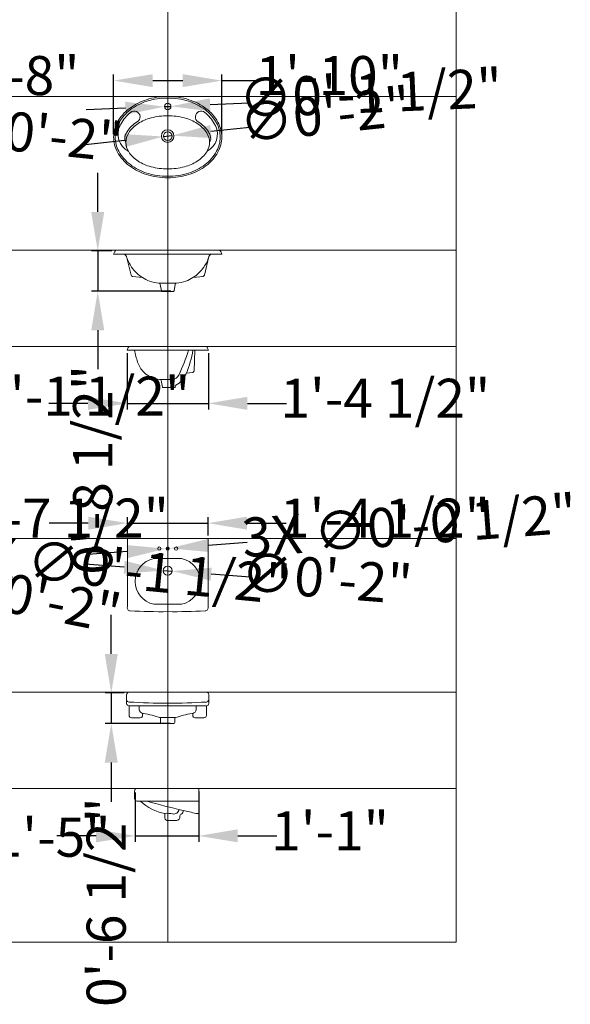
# Model space of a CAD drawing. Units: inches. Extents: x 2138 to 3265, y 2149 to 3392.
# Tile 12 of 13: x 3153 to 3265, y 3053 to 3255. Entities that reach past the tile are written whole.
import ezdxf

# ---------------------------------------------------------------- set-up
doc = ezdxf.new("R2010")
doc.units = ezdxf.units.IN
for name, color, linetype, lineweight in [('A-ANNO-DIMS', 2, 'Continuous', 18), ('A-DETL-GRID', 1, 'Continuous', 13), ('Washbasin-detail', 251, 'Continuous', 13), ('Washbasin-outline', 250, 'Continuous', 20)]:
    doc.layers.add(name, color=color, linetype=linetype, lineweight=lineweight)
doc.styles.get("Standard").update_dxf_attribs({"font": 'arial.ttf'})
doc.dimstyles.new('ISO-25', dxfattribs={"dimtxt": 8, "dimasz": 8, "dimexe": 1.25, "dimexo": 0.625, "dimtad": 0, "dimdec": 1, "dimlunit": 4, "dimtxsty": 'Standard', "dimcen": 2.5, "dimadec": 0, "dimazin": 0, "dimtfac": 1, "dimtdec": 1, "dimtmove": 0, "dimatfit": 3, "dimfxl": 1, "dimarcsym": 0})

# ---------------------------------------------------------------- blocks, each defined once
blk = doc.blocks.new('*D91')
at = {"layer": 'A-ANNO-DIMS', "color": 0, "lineweight": -2, "transparency": 16777216}
for p, q in [((3113.64, 3239.59), (3113.64, 3243.52)), ((3133.8, 3239.62), (3133.8, 3243.52)), ((3121.64, 3242.27), (3125.8, 3242.27)), ((3133.8, 3242.27), (3141.8, 3242.27))]:
    blk.add_line(p, q, dxfattribs=at)
at = {"layer": 'A-ANNO-DIMS', "color": 0, "transparency": 16777216}
for points in [[(3121.64, 3243.6), (3121.64, 3240.94), (3113.64, 3242.27)], [(3125.8, 3243.6), (3125.8, 3240.94), (3133.8, 3242.27)]]:
    blk.add_solid(points, dxfattribs=at)
at = {"layer": 'Defpoints', "color": 0, "transparency": 16777216}
for p in [(3133.8, 3242.27), (3113.64, 3238.97), (3133.8, 3239)]:
    blk.add_point(p, dxfattribs=at)
at = {"layer": 'A-ANNO-DIMS', "color": 0, "transparency": 16777216, "insert": (3152.69, 3242.27), "char_height": 8, "attachment_point": 5}
blk.add_mtext('1\'-8"', dxfattribs=at)
blk = doc.blocks.new('*D93')
at = {"layer": 'A-ANNO-DIMS', "color": 0, "lineweight": -2, "transparency": 16777216}
for p, q in [((3129.72, 3187.08), (3129.72, 3175.37)), ((3115.98, 3184.63), (3115.98, 3175.37)), ((3107.98, 3176.62), (3099.98, 3176.62)), ((3115.98, 3176.62), (3129.72, 3176.62)), ((3137.72, 3176.62), (3145.72, 3176.62))]:
    blk.add_line(p, q, dxfattribs=at)
at = {"layer": 'A-ANNO-DIMS', "color": 0, "transparency": 16777216}
for points in [[(3107.98, 3177.95), (3107.98, 3175.28), (3115.98, 3176.62)], [(3137.72, 3177.95), (3137.72, 3175.28), (3129.72, 3176.62)]]:
    blk.add_solid(points, dxfattribs=at)
at = {"layer": 'Defpoints', "color": 0, "transparency": 16777216}
for p in [(3129.72, 3187.71), (3115.98, 3185.26), (3129.72, 3176.62)]:
    blk.add_point(p, dxfattribs=at)
at = {"layer": 'A-ANNO-DIMS', "color": 0, "transparency": 16777216, "insert": (3165.92, 3176.62), "char_height": 8, "attachment_point": 5}
blk.add_mtext('1\'-1 1/2"', dxfattribs=at)
blk = doc.blocks.new('*D94')
at = {"layer": 'A-ANNO-DIMS', "color": 0, "lineweight": -2, "transparency": 16777216}
for p, q in [((3171.73, 3231.32), (3171.73, 3243.52)), ((3193.86, 3231.32), (3193.86, 3243.52)), ((3179.73, 3242.27), (3185.86, 3242.27)), ((3193.86, 3242.27), (3201.86, 3242.27))]:
    blk.add_line(p, q, dxfattribs=at)
at = {"layer": 'A-ANNO-DIMS', "color": 0, "transparency": 16777216}
for points in [[(3179.73, 3243.6), (3179.73, 3240.94), (3171.73, 3242.27)], [(3185.86, 3243.6), (3185.86, 3240.94), (3193.86, 3242.27)]]:
    blk.add_solid(points, dxfattribs=at)
at = {"layer": 'Defpoints', "color": 0, "transparency": 16777216}
for p in [(3193.86, 3242.27), (3171.73, 3230.69), (3193.86, 3230.69)]:
    blk.add_point(p, dxfattribs=at)
at = {"layer": 'A-ANNO-DIMS', "color": 0, "transparency": 16777216, "insert": (3215.85, 3242.27), "char_height": 8, "attachment_point": 5}
blk.add_mtext('1\'-10"', dxfattribs=at)
blk = doc.blocks.new('*D95')
at = {"layer": 'A-ANNO-DIMS', "color": 0, "lineweight": -2, "transparency": 16777216}
for p, q in [((3168.48, 3215.38), (3168.48, 3223.38)), ((3171.38, 3207.38), (3167.23, 3207.38)), ((3168.48, 3207.38), (3168.48, 3199.13)), ((3183.42, 3199.13), (3167.23, 3199.13)), ((3168.48, 3191.13), (3168.48, 3183.13))]:
    blk.add_line(p, q, dxfattribs=at)
at = {"layer": 'A-ANNO-DIMS', "color": 0, "transparency": 16777216}
for points in [[(3167.14, 3215.38), (3169.81, 3215.38), (3168.48, 3207.38)], [(3167.14, 3191.13), (3169.81, 3191.13), (3168.48, 3199.13)]]:
    blk.add_solid(points, dxfattribs=at)
at = {"layer": 'Defpoints', "color": 0, "transparency": 16777216}
for p in [(3172.01, 3207.38), (3168.48, 3199.13), (3184.05, 3199.13)]:
    blk.add_point(p, dxfattribs=at)
at = {"layer": 'A-ANNO-DIMS', "color": 0, "transparency": 16777216, "insert": (3168.48, 3162.55), "char_height": 8, "attachment_point": 5, "rotation": 90}
blk.add_mtext('0\'-8 1/2"', dxfattribs=at)
blk = doc.blocks.new('*D96')
at = {"layer": 'A-ANNO-DIMS', "color": 0, "lineweight": -2, "transparency": 16777216}
for p, q in [((3174.47, 3186.43), (3174.47, 3174.91)), ((3191.12, 3186.43), (3191.12, 3174.91)), ((3166.47, 3176.16), (3158.47, 3176.16)), ((3174.47, 3176.16), (3191.12, 3176.16)), ((3199.12, 3176.16), (3207.12, 3176.16))]:
    blk.add_line(p, q, dxfattribs=at)
at = {"layer": 'A-ANNO-DIMS', "color": 0, "transparency": 16777216}
for points in [[(3166.47, 3177.5), (3166.47, 3174.83), (3174.47, 3176.16)], [(3199.12, 3177.5), (3199.12, 3174.83), (3191.12, 3176.16)]]:
    blk.add_solid(points, dxfattribs=at)
at = {"layer": 'Defpoints', "color": 0, "transparency": 16777216}
for p in [(3174.47, 3187.05), (3191.12, 3187.05), (3191.12, 3176.16)]:
    blk.add_point(p, dxfattribs=at)
at = {"layer": 'A-ANNO-DIMS', "color": 0, "transparency": 16777216, "insert": (3227.32, 3176.16), "char_height": 8, "attachment_point": 5}
blk.add_mtext('1\'-4 1/2"', dxfattribs=at)
blk = doc.blocks.new('*D105')
at = {"layer": 'A-ANNO-DIMS', "color": 0, "lineweight": -2, "transparency": 16777216}
for p, q in [((3114.09, 3139.73), (3114.09, 3152.87)), ((3133.38, 3139.88), (3133.38, 3152.87)), ((3122.09, 3151.62), (3125.38, 3151.62)), ((3133.38, 3151.62), (3141.38, 3151.62))]:
    blk.add_line(p, q, dxfattribs=at)
at = {"layer": 'A-ANNO-DIMS', "color": 0, "transparency": 16777216}
for points in [[(3122.09, 3152.95), (3122.09, 3150.28), (3114.09, 3151.62)], [(3125.38, 3152.95), (3125.38, 3150.28), (3133.38, 3151.62)]]:
    blk.add_solid(points, dxfattribs=at)
at = {"layer": 'Defpoints', "color": 0, "transparency": 16777216}
for p in [(3133.38, 3151.62), (3114.09, 3139.11), (3133.38, 3139.26)]:
    blk.add_point(p, dxfattribs=at)
at = {"layer": 'A-ANNO-DIMS', "color": 0, "transparency": 16777216, "insert": (3161.58, 3151.62), "char_height": 8, "attachment_point": 5}
blk.add_mtext('1\'-7 1/2"', dxfattribs=at)
blk = doc.blocks.new('*D107')
at = {"layer": 'A-ANNO-DIMS', "color": 0, "lineweight": -2, "transparency": 16777216}
for p, q in [((3115.23, 3096.57), (3115.23, 3085.01)), ((3132.15, 3096.63), (3132.15, 3085.01)), ((3107.23, 3086.26), (3099.23, 3086.26)), ((3115.23, 3086.26), (3132.15, 3086.26)), ((3140.15, 3086.26), (3148.15, 3086.26))]:
    blk.add_line(p, q, dxfattribs=at)
at = {"layer": 'A-ANNO-DIMS', "color": 0, "transparency": 16777216}
for points in [[(3107.23, 3087.6), (3107.23, 3084.93), (3115.23, 3086.26)], [(3140.15, 3087.6), (3140.15, 3084.93), (3132.15, 3086.26)]]:
    blk.add_solid(points, dxfattribs=at)
at = {"layer": 'Defpoints', "color": 0, "transparency": 16777216}
for p in [(3115.23, 3097.2), (3132.15, 3097.25), (3132.15, 3086.26)]:
    blk.add_point(p, dxfattribs=at)
at = {"layer": 'A-ANNO-DIMS', "color": 0, "transparency": 16777216, "insert": (3159.03, 3086.26), "char_height": 8, "attachment_point": 5}
blk.add_mtext('1\'-5"', dxfattribs=at)
blk = doc.blocks.new('*D108')
at = {"layer": 'A-ANNO-DIMS', "color": 0, "lineweight": -2, "transparency": 16777216}
for p, q in [((3174.54, 3149.09), (3174.54, 3152.87)), ((3191.05, 3149.09), (3191.05, 3152.87)), ((3166.54, 3151.62), (3158.54, 3151.62)), ((3174.54, 3151.62), (3191.05, 3151.62)), ((3199.05, 3151.62), (3207.05, 3151.62))]:
    blk.add_line(p, q, dxfattribs=at)
at = {"layer": 'A-ANNO-DIMS', "color": 0, "transparency": 16777216}
for points in [[(3166.54, 3152.95), (3166.54, 3150.28), (3174.54, 3151.62)], [(3199.05, 3152.95), (3199.05, 3150.28), (3191.05, 3151.62)]]:
    blk.add_solid(points, dxfattribs=at)
at = {"layer": 'Defpoints', "color": 0, "transparency": 16777216}
for p in [(3191.05, 3151.62), (3174.54, 3148.47), (3191.05, 3148.47)]:
    blk.add_point(p, dxfattribs=at)
at = {"layer": 'A-ANNO-DIMS', "color": 0, "transparency": 16777216, "insert": (3227.25, 3151.62), "char_height": 8, "attachment_point": 5}
blk.add_mtext('1\'-4 1/2"', dxfattribs=at)
blk = doc.blocks.new('*D109')
at = {"layer": 'A-ANNO-DIMS', "color": 0, "lineweight": -2, "transparency": 16777216}
for p, q in [((3171.24, 3124.83), (3171.24, 3132.83)), ((3173.91, 3116.83), (3169.99, 3116.83)), ((3171.24, 3116.83), (3171.24, 3110.56)), ((3183.31, 3110.56), (3169.99, 3110.56)), ((3171.24, 3102.56), (3171.24, 3094.56))]:
    blk.add_line(p, q, dxfattribs=at)
at = {"layer": 'A-ANNO-DIMS', "color": 0, "transparency": 16777216}
for points in [[(3169.91, 3124.83), (3172.58, 3124.83), (3171.24, 3116.83)], [(3169.91, 3102.56), (3172.58, 3102.56), (3171.24, 3110.56)]]:
    blk.add_solid(points, dxfattribs=at)
at = {"layer": 'Defpoints', "color": 0, "transparency": 16777216}
for p in [(3174.54, 3116.83), (3171.24, 3110.56), (3183.93, 3110.56)]:
    blk.add_point(p, dxfattribs=at)
at = {"layer": 'A-ANNO-DIMS', "color": 0, "transparency": 16777216, "insert": (3171.24, 3073.99), "char_height": 8, "attachment_point": 5, "rotation": 90}
blk.add_mtext('0\'-6 1/2"', dxfattribs=at)
blk = doc.blocks.new('*D110')
at = {"layer": 'A-ANNO-DIMS', "color": 0, "lineweight": -2, "transparency": 16777216}
for p, q in [((3176.14, 3096.47), (3176.14, 3086.31)), ((3189.13, 3096.66), (3189.13, 3086.31)), ((3168.14, 3087.56), (3160.14, 3087.56)), ((3176.14, 3087.56), (3189.13, 3087.56)), ((3197.13, 3087.56), (3205.13, 3087.56))]:
    blk.add_line(p, q, dxfattribs=at)
at = {"layer": 'A-ANNO-DIMS', "color": 0, "transparency": 16777216}
for points in [[(3168.14, 3088.9), (3168.14, 3086.23), (3176.14, 3087.56)], [(3197.13, 3088.9), (3197.13, 3086.23), (3189.13, 3087.56)]]:
    blk.add_solid(points, dxfattribs=at)
at = {"layer": 'Defpoints', "color": 0, "transparency": 16777216}
for p in [(3176.14, 3097.1), (3189.13, 3097.29), (3189.13, 3087.56)]:
    blk.add_point(p, dxfattribs=at)
at = {"layer": 'A-ANNO-DIMS', "color": 0, "transparency": 16777216, "insert": (3216.01, 3087.56), "char_height": 8, "attachment_point": 5}
blk.add_mtext('1\'-1"', dxfattribs=at)
blk = doc.blocks.new('*D127')
at = {"layer": 'A-ANNO-DIMS', "color": 0, "lineweight": -2, "transparency": 16777216}
for p, q in [((3114.9, 3234.67), (3106.94, 3235.51)), ((3122.86, 3233.84), (3124.62, 3233.65)), ((3140.53, 3231.98), (3132.58, 3232.81))]:
    blk.add_line(p, q, dxfattribs=at)
at = {"layer": 'A-ANNO-DIMS', "color": 0, "transparency": 16777216}
for points in [[(3115.04, 3236), (3114.76, 3233.35), (3122.86, 3233.84)], [(3132.71, 3234.14), (3132.44, 3231.49), (3124.62, 3233.65)]]:
    blk.add_solid(points, dxfattribs=at)
at = {"layer": 'Defpoints', "color": 0, "transparency": 16777216}
for p in [(3122.86, 3233.84), (3124.62, 3233.65)]:
    blk.add_point(p, dxfattribs=at)
at = {"layer": 'A-ANNO-DIMS', "color": 0, "transparency": 16777216, "insert": (3156.06, 3230.35), "char_height": 8, "attachment_point": 5, "rotation": 353.9986}
blk.add_mtext('∅0\'-2"', dxfattribs=at)
blk = doc.blocks.new('*D128')
at = {"layer": 'A-ANNO-DIMS', "color": 0, "lineweight": -2, "transparency": 16777216}
for p, q in [((3199.45, 3237.66), (3191.46, 3237.33)), ((3174.13, 3236.61), (3166.14, 3236.29)), ((3182.12, 3236.94), (3183.46, 3237))]:
    blk.add_line(p, q, dxfattribs=at)
at = {"layer": 'A-ANNO-DIMS', "color": 0, "transparency": 16777216}
for points in [[(3174.08, 3237.95), (3174.19, 3235.28), (3182.12, 3236.94)], [(3191.4, 3238.66), (3191.51, 3236), (3183.46, 3237)]]:
    blk.add_solid(points, dxfattribs=at)
at = {"layer": 'Defpoints', "color": 0, "transparency": 16777216}
for p in [(3182.12, 3236.94), (3183.46, 3237)]:
    blk.add_point(p, dxfattribs=at)
at = {"layer": 'A-ANNO-DIMS', "color": 0, "transparency": 16777216, "insert": (3224.36, 3238.69), "char_height": 8, "attachment_point": 5, "rotation": 2.3614}
blk.add_mtext('∅0\'-1 1/2"', dxfattribs=at)
blk = doc.blocks.new('*D129')
at = {"layer": 'A-ANNO-DIMS', "color": 0, "lineweight": -2, "transparency": 16777216}
for p, q in [((3199.59, 3232.67), (3191.63, 3231.84)), ((3173.96, 3229.98), (3166, 3229.15)), ((3181.91, 3230.82), (3183.67, 3231))]:
    blk.add_line(p, q, dxfattribs=at)
at = {"layer": 'A-ANNO-DIMS', "color": 0, "transparency": 16777216}
for points in [[(3173.82, 3231.31), (3174.1, 3228.66), (3181.91, 3230.82)], [(3191.49, 3233.16), (3191.77, 3230.51), (3183.67, 3231)]]:
    blk.add_solid(points, dxfattribs=at)
at = {"layer": 'Defpoints', "color": 0, "transparency": 16777216}
for p in [(3181.91, 3230.82), (3183.67, 3231)]:
    blk.add_point(p, dxfattribs=at)
at = {"layer": 'A-ANNO-DIMS', "color": 0, "transparency": 16777216, "insert": (3215.11, 3234.3), "char_height": 8, "attachment_point": 5, "rotation": 5.9874}
blk.add_mtext('∅0\'-2"', dxfattribs=at)
blk = doc.blocks.new('*D136')
at = {"layer": 'A-ANNO-DIMS', "color": 0, "lineweight": -2, "transparency": 16777216}
for p, q in [((3115.11, 3146.91), (3107.15, 3147.69)), ((3123.07, 3146.13), (3124.4, 3146)), ((3140.33, 3144.45), (3132.37, 3145.22))]:
    blk.add_line(p, q, dxfattribs=at)
at = {"layer": 'A-ANNO-DIMS', "color": 0, "transparency": 16777216}
for points in [[(3115.24, 3148.24), (3114.98, 3145.58), (3123.07, 3146.13)], [(3132.5, 3146.55), (3132.24, 3143.9), (3124.4, 3146)]]:
    blk.add_solid(points, dxfattribs=at)
at = {"layer": 'Defpoints', "color": 0, "transparency": 16777216}
for p in [(3123.07, 3146.13), (3124.4, 3146)]:
    blk.add_point(p, dxfattribs=at)
at = {"layer": 'A-ANNO-DIMS', "color": 0, "transparency": 16777216, "insert": (3173.48, 3141.21), "char_height": 8, "attachment_point": 5, "rotation": 354.4214}
blk.add_mtext('3X ∅0\'-1 1/2"', dxfattribs=at)
blk = doc.blocks.new('*D137')
at = {"layer": 'A-ANNO-DIMS', "color": 0, "lineweight": -2, "transparency": 16777216}
for p, q in [((3115.02, 3143.3), (3107.17, 3144.86)), ((3122.87, 3141.75), (3124.61, 3141.41)), ((3140.3, 3138.3), (3132.46, 3139.85))]:
    blk.add_line(p, q, dxfattribs=at)
at = {"layer": 'A-ANNO-DIMS', "color": 0, "transparency": 16777216}
for points in [[(3115.28, 3144.61), (3114.76, 3142), (3122.87, 3141.75)], [(3132.71, 3141.16), (3132.2, 3138.55), (3124.61, 3141.41)]]:
    blk.add_solid(points, dxfattribs=at)
at = {"layer": 'Defpoints', "color": 0, "transparency": 16777216}
for p in [(3122.87, 3141.75), (3124.61, 3141.41)]:
    blk.add_point(p, dxfattribs=at)
at = {"layer": 'A-ANNO-DIMS', "color": 0, "transparency": 16777216, "insert": (3155.62, 3135.27), "char_height": 8, "attachment_point": 5, "rotation": 348.8088}
blk.add_mtext('∅0\'-2"', dxfattribs=at)
blk = doc.blocks.new('*D138')
at = {"layer": 'A-ANNO-DIMS', "color": 0, "lineweight": -2, "transparency": 16777216}
for p, q in [((3182.46, 3146.4), (3183.12, 3146.45)), ((3199.08, 3147.64), (3191.1, 3147.05)), ((3174.49, 3145.8), (3166.51, 3145.2))]:
    blk.add_line(p, q, dxfattribs=at)
at = {"layer": 'A-ANNO-DIMS', "color": 0, "transparency": 16777216}
for points in [[(3174.39, 3147.13), (3174.59, 3144.47), (3182.46, 3146.4)], [(3191, 3148.38), (3191.2, 3145.72), (3183.12, 3146.45)]]:
    blk.add_solid(points, dxfattribs=at)
at = {"layer": 'Defpoints', "color": 0, "transparency": 16777216}
for p in [(3183.12, 3146.45), (3182.46, 3146.4)]:
    blk.add_point(p, dxfattribs=at)
at = {"layer": 'A-ANNO-DIMS', "color": 0, "transparency": 16777216, "insert": (3232.29, 3150.13), "char_height": 8, "attachment_point": 5, "rotation": 4.2846}
blk.add_mtext('3X ∅0\'-0 1/2"', dxfattribs=at)
blk = doc.blocks.new('*D139')
at = {"layer": 'A-ANNO-DIMS', "color": 0, "lineweight": -2, "transparency": 16777216}
for p, q in [((3173.9, 3142.58), (3165.92, 3143.21)), ((3181.87, 3141.94), (3183.71, 3141.8)), ((3199.66, 3140.54), (3191.69, 3141.17))]:
    blk.add_line(p, q, dxfattribs=at)
at = {"layer": 'A-ANNO-DIMS', "color": 0, "transparency": 16777216}
for points in [[(3174, 3143.91), (3173.79, 3141.25), (3181.87, 3141.94)], [(3191.79, 3142.5), (3191.58, 3139.84), (3183.71, 3141.8)]]:
    blk.add_solid(points, dxfattribs=at)
at = {"layer": 'Defpoints', "color": 0, "transparency": 16777216}
for p in [(3181.87, 3141.94), (3183.71, 3141.8)]:
    blk.add_point(p, dxfattribs=at)
at = {"layer": 'A-ANNO-DIMS', "color": 0, "transparency": 16777216, "insert": (3215.23, 3139.3), "char_height": 8, "attachment_point": 5, "rotation": 355.4738}
blk.add_mtext('∅0\'-2"', dxfattribs=at)

msp = doc.modelspace()

# ---------------------------------------------------------------- linework, layer by layer
at = {"layer": 'A-DETL-GRID'}
for p, q in [((3182.79, 3239.02), (3182.79, 3370.91)), ((3241.85, 3239.02), (3241.85, 3370.91)), ((2828.46, 3239.02), (3241.85, 3239.02)), ((2828.46, 3239.02), (3241.85, 3239.02)), ((3182.79, 3148.47), (3182.79, 3239.02)), ((3241.85, 3148.47), (3241.85, 3239.02)), ((2828.46, 3207.52), (3241.85, 3207.52)), ((2828.46, 3187.84), (3241.85, 3187.84)), ((2828.46, 3148.47), (3241.85, 3148.47)), ((2828.46, 3148.47), (3241.85, 3148.47)), ((3182.79, 3065.79), (3182.79, 3148.47)), ((3241.85, 3065.79), (3241.85, 3148.47)), ((2828.46, 3116.97), (3241.85, 3116.97)), ((2828.46, 3097.29), (3241.85, 3097.29)), ((2828.46, 3065.79), (3241.85, 3065.79))]:
    msp.add_line(p, q, dxfattribs=at)
at = {"layer": 'Defpoints'}
msp.add_point((3182.79, 3224.18), dxfattribs=at)
at = {"layer": 'Washbasin-detail'}
for p, q in [((3175.3, 3202.42), (3174.36, 3206.23)), ((3190.29, 3202.42), (3191.23, 3206.23)), ((3175.56, 3202.18), (3177.63, 3201.92)), ((3190.03, 3202.18), (3187.96, 3201.92)), ((3181.05, 3200.75), (3182.79, 3200.75)), ((3184.54, 3200.75), (3182.79, 3200.75)), ((3181.19, 3181.08), (3183.66, 3181.08)), ((3182.79, 3111.79), (3181.21, 3111.79)), ((3182.79, 3111.79), (3184.38, 3111.79))]:
    msp.add_line(p, q, dxfattribs=at)
for points in [[(3182.79, 3238.7, 0.075684), (3178.53, 3238.05, 0.085949), (3175.16, 3236.33, 0.106021), (3172.79, 3233.6, 0.126461), (3172.04, 3230.69, 0.126461), (3172.79, 3227.79, 0.106021), (3175.16, 3225.06, 0.085949), (3178.53, 3223.33, 0.075684), (3182.79, 3222.68, 0.075684), (3187.06, 3223.33, 0.085949), (3190.43, 3225.06, 0.106021), (3192.8, 3227.79, 0.126461), (3193.54, 3230.69, 0.126461), (3192.8, 3233.6, 0.106021), (3190.43, 3236.33, 0.085949), (3187.06, 3238.05, 0.075684)], [(3182.79, 3135.01), (3179.95, 3135.01, -0.813225), (3179.95, 3144.38), (3182.79, 3144.38), (3185.63, 3144.38, -0.813225), (3185.63, 3135.01)]]:
    msp.add_lwpolyline(points, format="xyb", close=True, dxfattribs=at)
for points in [[(3173.04, 3233.05, -0.016104), (3173.2, 3233.37, -0.096892), (3175.21, 3235.77, -0.085949)], [(3192.55, 3233.05, 0.016104), (3192.38, 3233.37, 0.096892), (3190.38, 3235.77, 0.085949)], [(3174.09, 3231.03, -0.053872), (3174.48, 3231.79, -0.107172), (3176.53, 3233.82, -0.00132), (3176.57, 3233.84, -0.064562)], [(3191.49, 3231.03, 0.053872), (3191.11, 3231.79, 0.107172), (3189.06, 3233.82, 0.00132), (3189.02, 3233.84, 0.064562)], [(3182.79, 3114.72, -0.015438), (3174.88, 3114.98, -0.359652), (3174.39, 3115.43, 15.688123)], [(3182.79, 3114.72, 0.015438), (3190.71, 3114.98, 0.359652), (3191.19, 3115.43, -15.688123)], [(3177.26, 3094.66, 0.151862), (3182.22, 3092.16), (3182.22, 3091.24, 0.466229), (3182.84, 3090.72), (3184.6, 3090.72, 0.411247), (3185.29, 3091.54, -0.310137), (3185.56, 3092.01, 0.343594), (3185.94, 3092.77, 1.207474)], [(3182.22, 3092.16, -0.083549), (3183.8, 3092.06, 0.438642), (3185.09, 3092.97, -0.972265)]]:
    msp.add_lwpolyline(points, format="xyb", dxfattribs=at)
for centre, radius in [((3182.79, 3236.97), 0.669), ((3182.79, 3230.91), 0.886), ((3181.08, 3146.42), 0.33), ((3182.79, 3146.42), 0.33), ((3184.51, 3146.42), 0.33), ((3182.79, 3141.87), 0.923)]:
    msp.add_circle(centre, radius, dxfattribs=at)
for centre, radius, start, end in [((3175.95, 3234.85), 1.18, 301.4378, 129.0332), ((3189.63, 3234.85), 1.18, 50.9668, 238.5622), ((3176.56, 3231.29), 3.94, 153.4546, 242.2784), ((3182.79, 3230.91), 1.28, 90, 270), ((3182.79, 3230.91), 1.28, 270, 90), ((3189.02, 3231.29), 3.94, 297.7216, 26.5454), ((3175.55, 3230.44), 1.57, 158.0362, 212.9088), ((3190.03, 3230.44), 1.57, 327.0912, 21.9638), ((3175.6, 3202.49), 0.315, 193.7526, 262.7989), ((3189.99, 3202.49), 0.315, 277.2011, 346.2474), ((3156.73, 3195.7), 31.5, 334.1426, 344.0605), ((3168.47, 3189.99), 19.69, 337.0991, 351.4036), ((3183.66, 3182.65), 1.57, 270, 334.1426)]:
    msp.add_arc(centre, radius, start, end, dxfattribs=at)
at = {"layer": 'Washbasin-outline'}
for p, q in [((3171.73, 3206.74), (3171.95, 3207.28)), ((3172.31, 3207.52), (3182.79, 3207.52)), ((3193.27, 3207.52), (3182.79, 3207.52)), ((3193.86, 3206.74), (3193.64, 3207.28)), ((3171.73, 3206.74), (3173.68, 3206.74)), ((3173.68, 3206.74), (3182.79, 3206.74)), ((3191.9, 3206.74), (3182.79, 3206.74)), ((3193.86, 3206.74), (3191.9, 3206.74)), ((3181.5, 3199.2), (3181.26, 3200.51)), ((3181.61, 3199.1), (3182.79, 3199.1)), ((3183.97, 3199.1), (3182.79, 3199.1)), ((3184.09, 3199.2), (3184.32, 3200.51)), ((3174.68, 3187.59), (3174.47, 3187.05)), ((3176.01, 3187.05), (3174.47, 3187.05)), ((3175.05, 3187.84), (3190.54, 3187.84)), ((3187.94, 3187.05), (3176.01, 3187.05)), ((3187.94, 3187.05), (3191.12, 3187.05)), ((3188.18, 3182.79), (3188.36, 3187.05)), ((3191.12, 3187.05), (3190.9, 3187.59)), ((3181.71, 3179.51), (3181.48, 3180.82)), ((3187.91, 3182.49), (3186.6, 3182.33)), ((3181.83, 3179.41), (3184.19, 3179.41)), ((3184.31, 3179.51), (3184.33, 3179.67)), ((3189.13, 3097.29), (3189.13, 3094.66)), ((3189.13, 3092.14), (3189.13, 3094.66))]:
    msp.add_line(p, q, dxfattribs=at)
for points in [[(3182.79, 3239.02, 0.075684), (3178.43, 3238.36, 0.085949), (3174.97, 3236.58, 0.106021), (3172.51, 3233.75, 0.126461), (3171.73, 3230.69, 0.126461), (3172.51, 3227.64, 0.106021), (3174.97, 3224.8, 0.085949), (3178.43, 3223.03, 0.075684), (3182.79, 3222.37, 0.075684), (3187.15, 3223.03, 0.085949), (3190.62, 3224.8, 0.106021), (3193.07, 3227.64, 0.126461), (3193.86, 3230.69, 0.126461), (3193.07, 3233.75, 0.106021), (3190.62, 3236.58, 0.085949), (3187.15, 3238.36, 0.075684)], [(3182.79, 3148.47), (3174.54, 3148.47), (3174.54, 3134.48, 0.475742), (3175.14, 3133.63, 0.013082), (3182.79, 3133.49, 0.013082), (3190.45, 3133.63, 0.475742), (3191.05, 3134.48), (3191.05, 3148.47)]]:
    msp.add_lwpolyline(points, format="xyb", close=True, dxfattribs=at)
for points in [[(3182.79, 3224.18, -0.064562), (3179.38, 3224.62, -0.077438), (3176.74, 3225.77, -0.107172), (3174.81, 3227.69, -0.145186), (3174.23, 3229.63, -0.145186), (3174.81, 3231.57, -0.107172), (3176.74, 3233.49, -0.077438), (3179.38, 3234.64, -0.064562), (3182.79, 3235.08, -0.064562)], [(3182.79, 3224.18, 0.064562), (3186.21, 3224.62, 0.077438), (3188.85, 3225.77, 0.107172), (3190.78, 3227.69, 0.145186), (3191.36, 3229.63, 0.145186), (3190.78, 3231.57, 0.107172), (3188.85, 3233.49, 0.077438), (3186.21, 3234.64, 0.064562), (3182.79, 3235.08, 0.064562)], [(3182.79, 3116.97), (3174.88, 3116.97, 0.414214), (3174.39, 3116.49), (3174.39, 3114.69, 0.414214), (3174.88, 3114.21)], [(3182.79, 3116.97), (3190.71, 3116.97, -0.414214), (3191.19, 3116.49), (3191.19, 3114.69, -0.414214), (3190.71, 3114.21)], [(3174.88, 3114.21), (3182.79, 3114.21, 0.341127)], [(3177.67, 3112.64), (3177.67, 3112.25, -0.414214), (3177.19, 3111.76), (3175.36, 3111.76, -0.414214), (3174.88, 3112.25), (3174.88, 3114.21)], [(3177.67, 3112.64, -0.283122), (3176.96, 3113.41), (3176.96, 3114.21)], [(3190.71, 3114.21), (3182.79, 3114.21, -0.341127)], [(3187.92, 3112.64), (3187.92, 3112.25, 0.414214), (3188.4, 3111.76), (3190.22, 3111.76, 0.414214), (3190.71, 3112.25), (3190.71, 3114.21)], [(3187.92, 3112.64, 0.283122), (3188.63, 3113.41), (3188.63, 3114.21)], [(3182.79, 3110.56), (3181.66, 3110.56, -0.414214), (3181.32, 3110.9), (3181.32, 3111.76, 0.056607), (3177.81, 3112.61, -0.036401), (3177.67, 3112.64)], [(3182.79, 3110.56), (3183.93, 3110.56, 0.414214), (3184.27, 3110.9), (3184.27, 3111.76, -0.056607), (3187.77, 3112.61, 0.036401), (3187.92, 3112.64)], [(3189.13, 3097.29), (3176.46, 3097.29, 0.330224), (3175.99, 3096.75), (3175.99, 3095.2, 0.330224), (3176.46, 3094.66), (3177.26, 3094.66)], [(3178.51, 3094.66, 0.009641), (3185.94, 3092.77, 0.076865)], [(3185.94, 3092.77, 0.003428), (3188.6, 3092.16, 0.076865), (3189.13, 3092.14, -0.093006)]]:
    msp.add_lwpolyline(points, format="xyb", dxfattribs=at)
msp.add_lwpolyline([(3177.26, 3094.66), (3189.13, 3094.66)], dxfattribs=at)
for centre, radius, start, end in [((3172.31, 3207.13), 0.394, 90, 158.1986), ((3193.27, 3207.13), 0.394, 21.8014, 90), ((3173.68, 3206.03), 0.709, 17.0419, 90), ((3181.89, 3208.54), 7.87, 197.0419, 214.6702), ((3183.7, 3208.54), 7.87, 325.3298, 342.9581), ((3191.9, 3206.03), 0.709, 90, 162.9581), ((3181.89, 3208.54), 7.87, 214.6702, 237.2559), ((3183.7, 3208.54), 7.87, 302.7441, 325.3298), ((3181.89, 3208.54), 7.87, 237.2559, 249.0349), ((3181.47, 3207.44), 6.69, 249.0349, 265.7896), ((3184.12, 3207.44), 6.69, 274.2104, 290.9651), ((3183.7, 3208.54), 7.87, 290.9651, 302.7441), ((3180.95, 3200.45), 0.315, 10.1247, 85.7896), ((3181.61, 3199.22), 0.118, 190.1247, 270), ((3183.97, 3199.22), 0.118, 270, 349.8753), ((3184.63, 3200.45), 0.315, 94.2104, 169.8753), ((3175.05, 3187.44), 0.394, 90, 158.1986), ((3195.74, 3190.8), 20.08, 190.7493, 197.9539), ((3190.54, 3187.44), 0.394, 21.8014, 96.7604), ((3181.51, 3186.18), 5.12, 197.9539, 265.7947), ((3187.87, 3182.8), 0.315, 276.9212, 357.6932), ((3181.51, 3186.18), 5.12, 265.7947, 266.4387), ((3181.17, 3180.76), 0.315, 10.1247, 86.4387), ((3182.18, 3184.01), 4.72, 299.2305, 336.4265), ((3168.47, 3189.99), 19.69, 336.4265, 337.0991), ((3181.83, 3179.53), 0.118, 190.1247, 270), ((3184.19, 3179.53), 0.118, 270, 349.8753), ((3184.64, 3179.61), 0.315, 123.1426, 169.8753)]:
    msp.add_arc(centre, radius, start, end, dxfattribs=at)

# ---------------------------------------------------------------- dimensions: what is measured, and where the dimension line sits
at = {"layer": 'A-ANNO-DIMS'}
for p1, p2, picture, middle in [((3182.12, 3236.94), (3183.46, 3237), '*D128', (3224.36, 3238.69)), ((3181.91, 3230.82), (3183.67, 3231), '*D129', (3215.11, 3234.3)), ((3122.86, 3233.84), (3124.62, 3233.65), '*D127', (3156.06, 3230.35)), ((3122.87, 3141.75), (3124.61, 3141.41), '*D137', (3155.62, 3135.27)), ((3181.87, 3141.94), (3183.71, 3141.8), '*D139', (3215.23, 3139.3))]:
    dim = msp.add_diameter_dim_2p(p1=p1, p2=p2, dimstyle='ISO-25', override={"dimdec": 1, "dimlfac": 1, "dimrnd": 0, "dimzin": 1, "dimdsep": 46, "dimlunit": 4, "dimfrac": 2}, dxfattribs=at)
    dim.commit()
    dim.dimension.update_dxf_attribs({"geometry": picture, "text_midpoint": middle})
for base, p1, p2, picture, middle in [((3133.8, 3242.27), (3113.64, 3238.97), (3133.8, 3239), '*D91', (3152.69, 3242.27)), ((3193.86, 3242.27), (3171.73, 3230.69), (3193.86, 3230.69), '*D94', (3215.85, 3242.27)), ((3129.72, 3176.62), (3115.98, 3185.26), (3129.72, 3187.71), '*D93', (3165.92, 3176.62)), ((3191.1201, 3176.163), (3174.4666, 3187.0508), (3191.1201, 3187.0508), '*D96', (3227.3222, 3176.163)), ((3133.38, 3151.62), (3114.09, 3139.11), (3133.38, 3139.26), '*D105', (3161.58, 3151.62)), ((3191.05, 3151.62), (3174.54, 3148.47), (3191.05, 3148.47), '*D108', (3227.25, 3151.62)), ((3132.15, 3086.26), (3115.23, 3097.2), (3132.15, 3097.25), '*D107', (3159.03, 3086.26)), ((3189.13, 3087.56), (3176.14, 3097.1), (3189.13, 3097.29), '*D110', (3216.01, 3087.56))]:
    dim = msp.add_linear_dim(base=base, p1=p1, p2=p2, dimstyle='ISO-25', override={"dimdec": 1, "dimlfac": 1, "dimrnd": 0, "dimzin": 1, "dimdsep": 46, "dimlunit": 4, "dimfrac": 2}, dxfattribs=at)
    dim.commit()
    dim.dimension.update_dxf_attribs({"geometry": picture, "text_midpoint": middle})
for base, p1, p2, picture, middle in [((3168.4782, 3199.1256), (3172.006, 3207.3775), (3184.0498, 3199.1256), '*D95', (3168.4782, 3162.547)), ((3171.24, 3110.56), (3174.54, 3116.83), (3183.93, 3110.56), '*D109', (3171.24, 3073.99))]:
    dim = msp.add_linear_dim(base=base, p1=p1, p2=p2, angle=90, dimstyle='ISO-25', override={"dimdec": 1, "dimlfac": 1, "dimrnd": 0, "dimzin": 1, "dimdsep": 46, "dimlunit": 4, "dimfrac": 2}, dxfattribs=at)
    dim.commit()
    dim.dimension.update_dxf_attribs({"geometry": picture, "text_midpoint": middle})
for p1, p2, picture, middle in [((3182.46, 3146.4), (3183.12, 3146.45), '*D138', (3232.29, 3150.13)), ((3123.07, 3146.13), (3124.4, 3146), '*D136', (3173.48, 3141.21))]:
    dim = msp.add_diameter_dim_2p(p1=p1, p2=p2, text='3X <>', dimstyle='ISO-25', override={"dimdec": 1, "dimlfac": 1, "dimrnd": 0, "dimzin": 1, "dimdsep": 46, "dimlunit": 4, "dimfrac": 2}, dxfattribs=at)
    dim.commit()
    dim.dimension.update_dxf_attribs({"geometry": picture, "text_midpoint": middle, "dimtype": 163})

doc.saveas('drawing.dxf')
